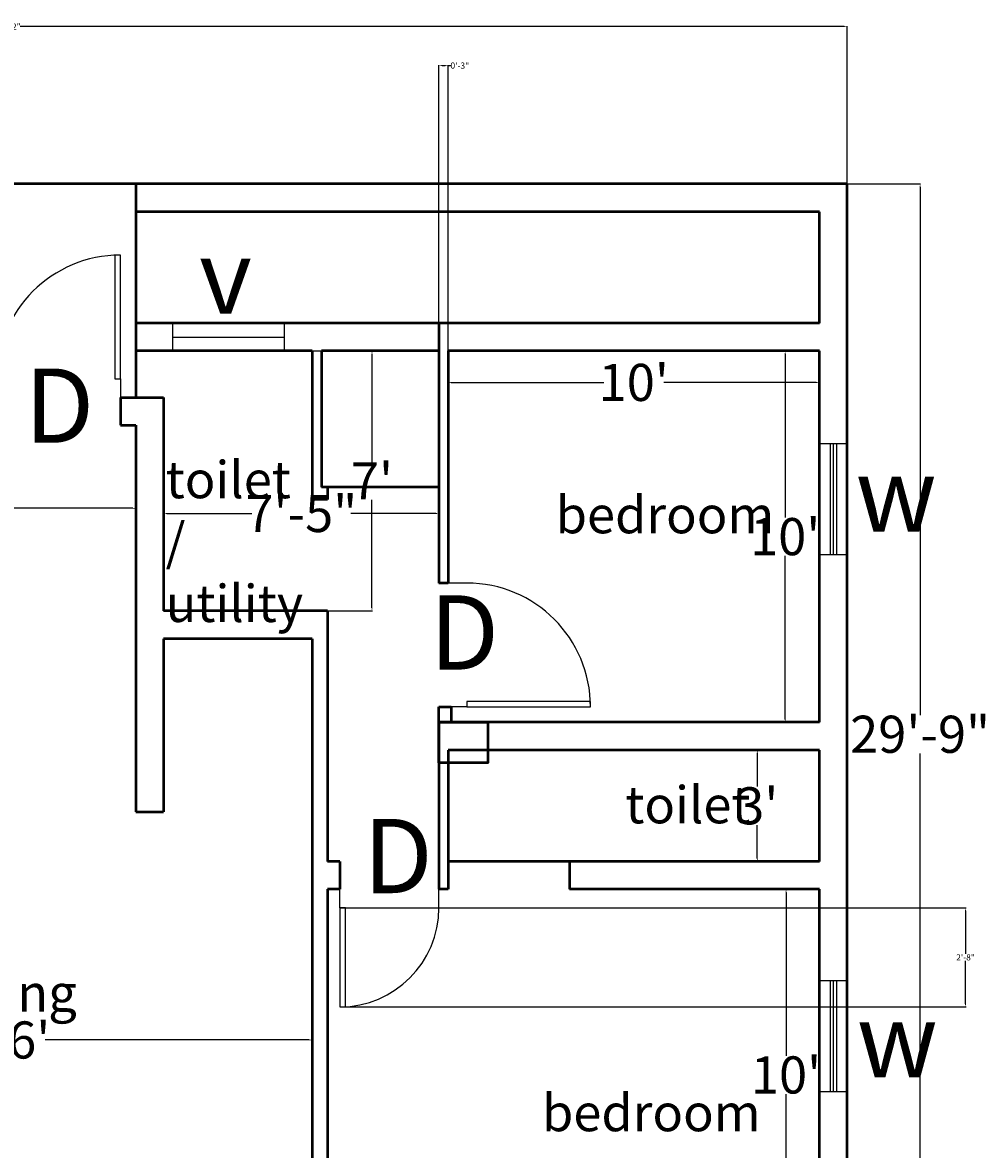
# Model space of a CAD drawing. Units: inches. Extents: x 409 to 7572, y 7 to 725.
# Tile 13 of 38: x 1972 to 2283, y 360 to 725. Entities that reach past the tile are written whole.
import ezdxf

# ---------------------------------------------------------------- set-up
doc = ezdxf.new("R2010")
doc.units = ezdxf.units.IN
doc.header["$MEASUREMENT"] = 0
for name, color, linetype, lineweight in [('A-ANNO-DIMS', 2, 'Continuous', 18), ('A-ANNO-SYMB', 3, 'Continuous', 25), ('A-AREA-IDEN', 7, 'Continuous', 25), ('A-DOOR', 3, 'Continuous', 25), ('A-GLAZ', 4, 'Continuous', 25), ('A-WALL', 7, 'Continuous', 50)]:
    doc.layers.add(name, color=color, linetype=linetype, lineweight=lineweight)
doc.styles.get("Standard").update_dxf_attribs({"font": 'arial.ttf'})
doc.dimstyles.get("Standard").update_dxf_attribs({"dimtxt": 2, "dimasz": 1, "dimexe": 0.18, "dimexo": 0.0625, "dimgap": 0.09, "dimtad": 0, "dimtih": 1, "dimtoh": 1, "dimdec": 0, "dimzin": 0, "dimdsep": 46, "dimlunit": 3, "dimtxsty": 'Standard', "dimcen": 0.09, "dimadec": 0, "dimazin": 0, "dimtfac": 1, "dimtdec": 0, "dimtofl": 0, "dimtmove": 0, "dimatfit": 3, "dimfxl": 1, "dimtolj": 1, "dimtzin": 0, "dimarcsym": 0})

# ---------------------------------------------------------------- blocks, each defined once
blk = doc.blocks.new('*U2')
for p, q in [((0, 0), (0, -6)), ((-40, 0), (-40, -6))]:
    blk.add_line(p, q)
blk.add_lwpolyline([(0, 0), (0, 40), (-1.75, 40), (-1.75, 0)], close=True)
blk.add_arc((0, 0), 40, 90, 180)
blk = doc.blocks.new('*U6')
for p, q in [((0, 0), (0, -6)), ((-40, 0), (-40, -6))]:
    blk.add_line(p, q)
blk.add_lwpolyline([(0, 0), (0, 40), (-1.75, 40), (-1.75, 0)], close=True)
blk.add_arc((0, 0), 40, 90, 180)
blk = doc.blocks.new('*U7')
for p, q in [((0, 0), (0, 6)), ((32, 0), (32, 6))]:
    blk.add_line(p, q)
blk.add_lwpolyline([(0, 0), (0, -32), (1.75, -32), (1.75, 0)], close=True)
blk.add_arc((0, 0), 32, 270, 0)
blk = doc.blocks.new('*D45')
at = {"layer": 'A-ANNO-DIMS', "color": 0, "lineweight": -2, "transparency": 16777216}
for p, q in [((2109.32, 618.47), (2109.32, 608.19)), ((2229.32, 618.47), (2229.32, 608.19)), ((2110.32, 608.37), (2159.61, 608.37)), ((2228.32, 608.37), (2179.03, 608.37))]:
    blk.add_line(p, q, dxfattribs=at)
at = {"layer": 'A-ANNO-DIMS', "color": 0, "transparency": 16777216}
for points in [[(2110.32, 608.54), (2110.32, 608.2), (2109.32, 608.37)], [(2228.32, 608.54), (2228.32, 608.2), (2229.32, 608.37)]]:
    blk.add_solid(points, dxfattribs=at)
at = {"layer": 'DEFPOINTS', "color": 0, "transparency": 16777216}
for p in [(2109.32, 618.53), (2229.32, 618.53), (2109.32, 608.37)]:
    blk.add_point(p, dxfattribs=at)
at = {"layer": 'A-ANNO-DIMS', "color": 0, "transparency": 16777216, "insert": (2169.32, 608.37), "char_height": 2, "attachment_point": 5}
blk.add_mtext("\\A1;{\\H6x;10'}", dxfattribs=at)
blk = doc.blocks.new('*D46')
at = {"layer": 'A-ANNO-DIMS', "color": 0, "lineweight": -2, "transparency": 16777216}
for p, q in [((2229.26, 618.53), (2218.09, 618.53)), ((2218.27, 617.53), (2218.27, 564.75)), ((2218.27, 499.53), (2218.27, 552.31)), ((2229.26, 498.53), (2218.09, 498.53))]:
    blk.add_line(p, q, dxfattribs=at)
at = {"layer": 'A-ANNO-DIMS', "color": 0, "transparency": 16777216}
for points in [[(2218.1, 617.53), (2218.43, 617.53), (2218.27, 618.53)], [(2218.1, 499.53), (2218.43, 499.53), (2218.27, 498.53)]]:
    blk.add_solid(points, dxfattribs=at)
at = {"layer": 'DEFPOINTS', "color": 0, "transparency": 16777216}
for p in [(2218.27, 618.53), (2229.32, 618.53), (2229.32, 498.53)]:
    blk.add_point(p, dxfattribs=at)
at = {"layer": 'A-ANNO-DIMS', "color": 0, "transparency": 16777216, "insert": (2218.27, 558.53), "char_height": 2, "attachment_point": 5}
blk.add_mtext("\\A1;{\\H6x;10'}", dxfattribs=at)
blk = doc.blocks.new('*D47')
at = {"layer": 'A-ANNO-DIMS', "color": 0, "lineweight": -2, "transparency": 16777216}
for p, q in [((2229.26, 444.53), (2218.37, 444.53)), ((2218.55, 443.53), (2218.55, 390.75)), ((2218.55, 325.53), (2218.55, 378.31)), ((2229.26, 324.53), (2218.37, 324.53))]:
    blk.add_line(p, q, dxfattribs=at)
at = {"layer": 'A-ANNO-DIMS', "color": 0, "transparency": 16777216}
for points in [[(2218.39, 443.53), (2218.72, 443.53), (2218.55, 444.53)], [(2218.39, 325.53), (2218.72, 325.53), (2218.55, 324.53)]]:
    blk.add_solid(points, dxfattribs=at)
at = {"layer": 'DEFPOINTS', "color": 0, "transparency": 16777216}
for p in [(2218.55, 444.53), (2229.32, 444.53), (2229.32, 324.53)]:
    blk.add_point(p, dxfattribs=at)
at = {"layer": 'A-ANNO-DIMS', "color": 0, "transparency": 16777216, "insert": (2218.55, 384.53), "char_height": 2, "attachment_point": 5}
blk.add_mtext("\\A1;{\\H6x;10'}", dxfattribs=at)
blk = doc.blocks.new('*D51')
at = {"layer": 'A-ANNO-DIMS', "color": 0, "lineweight": -2, "transparency": 16777216}
for p, q in [((1873.32, 563.4), (1873.32, 567.87)), ((1874.32, 567.69), (1920.68, 567.69)), ((2007.32, 567.69), (1960.96, 567.69)), ((2008.32, 563.4), (2008.32, 567.87))]:
    blk.add_line(p, q, dxfattribs=at)
at = {"layer": 'A-ANNO-DIMS', "color": 0, "transparency": 16777216}
for points in [[(1874.32, 567.86), (1874.32, 567.52), (1873.32, 567.69)], [(2007.32, 567.86), (2007.32, 567.52), (2008.32, 567.69)]]:
    blk.add_solid(points, dxfattribs=at)
at = {"layer": 'DEFPOINTS', "color": 0, "transparency": 16777216}
for p in [(2008.32, 567.69), (1873.32, 563.33), (2008.32, 563.33)]:
    blk.add_point(p, dxfattribs=at)
at = {"layer": 'A-ANNO-DIMS', "color": 0, "transparency": 16777216, "insert": (1940.82, 567.69), "char_height": 2, "attachment_point": 5}
blk.add_mtext('\\A1;{\\H6x;11\'-3"}', dxfattribs=at)
blk = doc.blocks.new('*D52')
at = {"layer": 'A-ANNO-DIMS', "color": 0, "lineweight": -2, "transparency": 16777216}
for p, q in [((1873.32, 403.47), (1873.32, 395.65)), ((2065.32, 403.47), (2065.32, 395.65)), ((1874.32, 395.83), (1959.61, 395.83)), ((2064.32, 395.83), (1979.03, 395.83))]:
    blk.add_line(p, q, dxfattribs=at)
at = {"layer": 'A-ANNO-DIMS', "color": 0, "transparency": 16777216}
for points in [[(1874.32, 396), (1874.32, 395.66), (1873.32, 395.83)], [(2064.32, 396), (2064.32, 395.66), (2065.32, 395.83)]]:
    blk.add_solid(points, dxfattribs=at)
at = {"layer": 'DEFPOINTS', "color": 0, "transparency": 16777216}
for p in [(1873.32, 403.53), (2065.32, 403.53), (2065.32, 395.83)]:
    blk.add_point(p, dxfattribs=at)
at = {"layer": 'A-ANNO-DIMS', "color": 0, "transparency": 16777216, "insert": (1969.32, 395.83), "char_height": 2, "attachment_point": 5}
blk.add_mtext("\\A1;{\\H6x;16'}", dxfattribs=at)
blk = doc.blocks.new('*D57')
at = {"layer": 'A-ANNO-DIMS', "color": 0, "lineweight": -2, "transparency": 16777216}
for p, q in [((2017.32, 568.97), (2017.32, 565.83)), ((2106.32, 568.97), (2106.32, 565.83)), ((2018.32, 566.01), (2045.83, 566.01)), ((2105.32, 566.01), (2077.81, 566.01))]:
    blk.add_line(p, q, dxfattribs=at)
at = {"layer": 'A-ANNO-DIMS', "color": 0, "transparency": 16777216}
for points in [[(2018.32, 566.17), (2018.32, 565.84), (2017.32, 566.01)], [(2105.32, 566.17), (2105.32, 565.84), (2106.32, 566.01)]]:
    blk.add_solid(points, dxfattribs=at)
at = {"layer": 'DEFPOINTS', "color": 0, "transparency": 16777216}
for p in [(2017.32, 569.03), (2106.32, 569.03), (2106.32, 566.01)]:
    blk.add_point(p, dxfattribs=at)
at = {"layer": 'A-ANNO-DIMS', "color": 0, "transparency": 16777216, "insert": (2061.82, 566.01), "char_height": 2, "attachment_point": 5}
blk.add_mtext('\\A1;{\\H6x;7\'-5"}', dxfattribs=at)
blk = doc.blocks.new('*D58')
at = {"layer": 'A-ANNO-DIMS', "color": 0, "lineweight": -2, "transparency": 16777216}
for p, q in [((2036.88, 618.53), (2084.86, 618.53)), ((2084.68, 617.53), (2084.68, 582.62)), ((2084.68, 535.53), (2084.68, 570.44)), ((2036.88, 534.53), (2084.86, 534.53))]:
    blk.add_line(p, q, dxfattribs=at)
at = {"layer": 'A-ANNO-DIMS', "color": 0, "transparency": 16777216}
for points in [[(2084.51, 617.53), (2084.84, 617.53), (2084.68, 618.53)], [(2084.51, 535.53), (2084.84, 535.53), (2084.68, 534.53)]]:
    blk.add_solid(points, dxfattribs=at)
at = {"layer": 'DEFPOINTS', "color": 0, "transparency": 16777216}
for p in [(2036.82, 618.53), (2036.82, 534.53), (2084.68, 534.53)]:
    blk.add_point(p, dxfattribs=at)
at = {"layer": 'A-ANNO-DIMS', "color": 0, "transparency": 16777216, "insert": (2084.68, 576.53), "char_height": 2, "attachment_point": 5}
blk.add_mtext("\\A1;{\\H6x;7'}", dxfattribs=at)
blk = doc.blocks.new('*D60')
at = {"layer": 'A-ANNO-DIMS', "color": 0, "lineweight": -2, "transparency": 16777216}
for p, q in [((2229.26, 489.53), (2209.07, 489.53)), ((2209.25, 488.53), (2209.25, 477.75)), ((2209.25, 454.53), (2209.25, 465.31)), ((2229.26, 453.53), (2209.07, 453.53))]:
    blk.add_line(p, q, dxfattribs=at)
at = {"layer": 'A-ANNO-DIMS', "color": 0, "transparency": 16777216}
for points in [[(2209.08, 488.53), (2209.41, 488.53), (2209.25, 489.53)], [(2209.08, 454.53), (2209.41, 454.53), (2209.25, 453.53)]]:
    blk.add_solid(points, dxfattribs=at)
at = {"layer": 'DEFPOINTS', "color": 0, "transparency": 16777216}
for p in [(2229.32, 489.53), (2209.25, 453.53), (2229.32, 453.53)]:
    blk.add_point(p, dxfattribs=at)
at = {"layer": 'A-ANNO-DIMS', "color": 0, "transparency": 16777216, "insert": (2209.25, 471.53), "char_height": 2, "attachment_point": 5}
blk.add_mtext("\\A1;{\\H6x;3'}", dxfattribs=at)
blk = doc.blocks.new('*D62')
at = {"layer": 'A-ANNO-DIMS', "color": 0, "lineweight": -2, "transparency": 16777216}
for p, q in [((1696.32, 672.59), (1696.32, 723.56)), ((1697.32, 723.38), (1963.75, 723.38)), ((2237.32, 723.38), (1970.88, 723.38)), ((2238.32, 672.59), (2238.32, 723.56))]:
    blk.add_line(p, q, dxfattribs=at)
at = {"layer": 'A-ANNO-DIMS', "color": 0, "transparency": 16777216}
for points in [[(1697.32, 723.55), (1697.32, 723.22), (1696.32, 723.38)], [(2237.32, 723.55), (2237.32, 723.22), (2238.32, 723.38)]]:
    blk.add_solid(points, dxfattribs=at)
at = {"layer": 'DEFPOINTS', "color": 0, "transparency": 16777216}
for p in [(1696.32, 723.38), (1696.32, 672.53), (2238.32, 672.53)]:
    blk.add_point(p, dxfattribs=at)
at = {"layer": 'A-ANNO-DIMS', "color": 0, "transparency": 16777216, "insert": (1967.32, 723.38), "char_height": 2, "attachment_point": 5}
blk.add_mtext('\\A1;45\'-2"', dxfattribs=at)
blk = doc.blocks.new('*D64')
at = {"layer": 'A-ANNO-DIMS', "color": 0, "lineweight": -2, "transparency": 16777216}
for p, q in [((2238.38, 672.53), (2262.07, 672.53)), ((2261.89, 671.53), (2261.89, 500.86)), ((2261.89, 316.53), (2261.89, 488.43)), ((2238.38, 315.53), (2262.07, 315.53))]:
    blk.add_line(p, q, dxfattribs=at)
at = {"layer": 'A-ANNO-DIMS', "color": 0, "transparency": 16777216}
for points in [[(2261.72, 671.53), (2262.05, 671.53), (2261.89, 672.53)], [(2261.72, 316.53), (2262.05, 316.53), (2261.89, 315.53)]]:
    blk.add_solid(points, dxfattribs=at)
at = {"layer": 'DEFPOINTS', "color": 0, "transparency": 16777216}
for p in [(2238.32, 672.53), (2261.89, 672.53), (2238.32, 315.53)]:
    blk.add_point(p, dxfattribs=at)
at = {"layer": 'A-ANNO-DIMS', "color": 0, "transparency": 16777216, "insert": (2261.89, 494.65), "char_height": 2, "attachment_point": 5}
blk.add_mtext('\\A1;{\\H6x;29\'-9"}', dxfattribs=at)
blk = doc.blocks.new('WIN-36')
for p, q in [((1699.82, 514.65), (1699.82, 478.65)), ((1700.82, 514.65), (1700.82, 478.65)), ((1701.82, 514.65), (1701.82, 478.65))]:
    blk.add_line(p, q)
blk.add_lwpolyline([(1705.32, 514.65), (1705.32, 478.65), (1696.32, 478.65), (1696.32, 514.65)], close=True)
blk = doc.blocks.new('VENT-36')
blk.add_line((5633.28, 355.73), (5633.28, 391.73))
blk.add_lwpolyline([(5628.78, 355.73), (5628.78, 391.73), (5637.78, 391.73), (5637.78, 355.73)], close=True)
blk = doc.blocks.new('*D180')
at = {"layer": 'A-ANNO-DIMS', "color": 0, "lineweight": -2, "transparency": 16777216}
for p, q in [((2106.32, 627.59), (2106.32, 710.96)), ((2107.32, 710.78), (2108.32, 710.78)), ((2109.32, 618.59), (2109.32, 710.96)), ((2109.32, 710.78), (2110.32, 710.78))]:
    blk.add_line(p, q, dxfattribs=at)
at = {"layer": 'A-ANNO-DIMS', "color": 0, "transparency": 16777216}
for points in [[(2107.32, 710.95), (2107.32, 710.61), (2106.32, 710.78)], [(2108.32, 710.95), (2108.32, 710.61), (2109.32, 710.78)]]:
    blk.add_solid(points, dxfattribs=at)
at = {"layer": 'DEFPOINTS', "color": 0, "transparency": 16777216}
for p in [(2109.32, 710.78), (2106.32, 627.53), (2109.32, 618.53)]:
    blk.add_point(p, dxfattribs=at)
at = {"layer": 'A-ANNO-DIMS', "color": 0, "transparency": 16777216, "insert": (2113.07, 710.78), "char_height": 2, "attachment_point": 5}
blk.add_mtext('\\A1;0\'-3"', dxfattribs=at)
blk = doc.blocks.new('*D181')
at = {"layer": 'A-ANNO-DIMS', "color": 0, "lineweight": -2, "transparency": 16777216}
for p, q in [((2074.38, 438.53), (2276.75, 438.53)), ((2276.57, 437.53), (2276.57, 423.64)), ((2276.57, 407.53), (2276.57, 421.42)), ((2074.38, 406.53), (2276.75, 406.53))]:
    blk.add_line(p, q, dxfattribs=at)
at = {"layer": 'A-ANNO-DIMS', "color": 0, "transparency": 16777216}
for points in [[(2276.4, 437.53), (2276.74, 437.53), (2276.57, 438.53)], [(2276.4, 407.53), (2276.74, 407.53), (2276.57, 406.53)]]:
    blk.add_solid(points, dxfattribs=at)
at = {"layer": 'DEFPOINTS', "color": 0, "transparency": 16777216}
for p in [(2074.32, 438.53), (2074.32, 406.53), (2276.57, 406.53)]:
    blk.add_point(p, dxfattribs=at)
at = {"layer": 'A-ANNO-DIMS', "color": 0, "transparency": 16777216, "insert": (2276.57, 422.53), "char_height": 2, "attachment_point": 5}
blk.add_mtext('\\A1;2\'-8"', dxfattribs=at)

msp = doc.modelspace()

# ---------------------------------------------------------------- linework, layer by layer
at = {"layer": 'A-WALL'}
for p, q in [((2238.32, 672.53), (1696.32, 672.53)), ((2008.32, 672.53), (2008.32, 603.53)), ((2238.32, 315.53), (2238.32, 672.53)), ((2229.32, 663.53), (2008.32, 663.53)), ((2229.32, 627.53), (2229.32, 663.53)), ((2229.32, 627.53), (2008.32, 627.53)), ((2106.32, 627.53), (2106.32, 543.53)), ((2065.32, 618.53), (2008.32, 618.53)), ((2065.32, 618.53), (2065.32, 570.53)), ((2106.32, 618.53), (2068.32, 618.53)), ((2068.32, 618.53), (2068.32, 574.53)), ((2229.32, 618.53), (2109.32, 618.53)), ((2109.32, 618.53), (2109.32, 543.53)), ((2229.32, 498.53), (2229.32, 618.53)), ((2003.32, 603.53), (2017.32, 603.53)), ((2003.32, 603.53), (2003.32, 594.53)), ((2017.32, 603.53), (2017.32, 534.53)), ((2003.32, 594.53), (2008.32, 594.53)), ((2106.32, 574.53), (2068.32, 574.53)), ((2070.32, 574.53), (2070.32, 570.53)), ((2070.32, 570.53), (2065.32, 570.53)), ((2109.32, 543.53), (2106.32, 543.53)), ((2070.32, 534.53), (2017.32, 534.53)), ((2070.32, 534.53), (2070.32, 453.53)), ((2065.32, 525.53), (2017.32, 525.53)), ((2017.32, 525.53), (2017.32, 469.53)), ((2065.32, 525.53), (2065.32, 337.53)), ((2106.32, 498.53), (2106.32, 503.53)), ((2106.32, 503.53), (2110.32, 503.53)), ((2110.32, 503.53), (2110.32, 498.53)), ((2229.32, 498.53), (2106.32, 498.53)), ((2106.32, 498.53), (2106.32, 444.53)), ((2065.32, 489.53), (2065.32, 337.53)), ((2229.32, 489.53), (2109.32, 489.53)), ((2109.32, 489.53), (2109.32, 444.53)), ((2229.32, 453.53), (2229.32, 489.53)), ((2008.32, 469.53), (2017.32, 469.53)), ((2074.32, 453.53), (2070.32, 453.53)), ((2074.32, 453.53), (2074.32, 444.53)), ((2229.32, 453.53), (2109.32, 453.53)), ((2148.51, 453.53), (2148.51, 444.53)), ((2074.32, 444.53), (2070.32, 444.53)), ((2070.32, 444.53), (2070.32, 324.53)), ((2109.32, 444.53), (2106.32, 444.53)), ((2109.32, 444.53), (2106.32, 444.53)), ((2229.32, 444.53), (2148.51, 444.53)), ((2229.32, 324.53), (2229.32, 444.53))]:
    msp.add_line(p, q, dxfattribs=at)
msp.add_lwpolyline([(2008.32, 594.53), (2008.32, 525.53), (2008.32, 469.53)], dxfattribs=at)
msp.add_lwpolyline([(2106.32, 498.53), (2122.18, 498.53), (2122.18, 485.36), (2106.32, 485.36)], close=True, dxfattribs=at)

# ---------------------------------------------------------------- block references
at = {"layer": 'A-DOOR'}
for name, p in [('*U2', (2003.32, 609.53)), ('*U7', (2074.32, 438.53))]:
    msp.add_blockref(name, p, dxfattribs=at)
at = {"layer": 'A-DOOR', "rotation": 270}
msp.add_blockref('*U6', (2115.32, 503.53), dxfattribs=at)
at = {"layer": 'A-GLAZ', "rotation": 269.9999999999996}
msp.add_blockref('VENT-36', (1664.51, 6256.31), dxfattribs=at)
at = {"layer": 'A-GLAZ'}
for p in [(533, 73.99), (533, -99.57)]:
    msp.add_blockref('WIN-36', p, dxfattribs=at)

# ---------------------------------------------------------------- texts
at = {"layer": 'A-ANNO-SYMB', "char_height": 24, "attachment_point": 1}
for s, width, insert in [('v', 18.2582, (2028.79, 654.55)), ('D', 19.1972, (1972.35, 612.87)), ('w', 18.2582, (2241, 584.1)), ('D', 19.1972, (2103.25, 539.54)), ('D', 19.1972, (2081.82, 467.28)), ('w', 18.2582, (2241.38, 407.81))]:
    msp.add_mtext_dynamic_manual_height_columns(s, width=width, gutter_width=1, heights=[0], dxfattribs=dict(at, insert=insert))
at = {"layer": 'A-AREA-IDEN', "char_height": 12, "attachment_point": 1}
for s, width, insert in [('toilet / utility', 49.2946, (2017.97, 582.94)), ('bedroom', 40.9017, (2144.07, 571.6)), ('toilet', 49.2946, (2166.57, 477.86)), ('Dining ', 67.5069, (1939.75, 417.03)), ('bedroom', 40.9017, (2139.65, 378.34))]:
    msp.add_mtext_dynamic_manual_height_columns(s, width=width, gutter_width=1, heights=[0], dxfattribs=dict(at, insert=insert))

# ---------------------------------------------------------------- dimensions: what is measured, and where the dimension line sits
at = {"layer": 'A-ANNO-DIMS'}
for base, p1, p2, override, picture, middle in [((1696.32, 723.38), (2238.32, 672.53), (1696.32, 672.53), {"dimclrd": 0, "dimclre": 0, "dimclrt": 0}, '*D62', (1967.32, 723.38)), ((2109.32, 710.78), (2106.32, 627.53), (2109.32, 618.53), {"dimdec": 1, "dimlfac": 1, "dimrnd": 0, "dimzin": 1, "dimdsep": 46, "dimlunit": 4, "dimfrac": 2}, '*D180', (2113.07, 710.78))]:
    dim = msp.add_linear_dim(base=base, p1=p1, p2=p2, dimstyle='Standard', override=override, dxfattribs=at)
    dim.commit()
    dim.dimension.update_dxf_attribs({"geometry": picture, "text_midpoint": middle})
dim = msp.add_linear_dim(base=(2261.89, 672.53), p1=(2238.32, 315.53), p2=(2238.32, 672.53), angle=90, text='{\\H6x;<>}', dimstyle='Standard', override={"dimclrd": 0, "dimclre": 0, "dimclrt": 0}, dxfattribs=at)
dim.commit()
dim.dimension.update_dxf_attribs({"geometry": '*D64', "text_midpoint": (2261.89, 494.65), "dimtype": 160})
for base, p1, p2, picture, middle in [((2084.68, 534.53), (2036.82, 618.53), (2036.82, 534.53), '*D58', (2084.68, 576.53)), ((2218.27, 618.53), (2229.32, 498.53), (2229.32, 618.53), '*D46', (2218.27, 558.53)), ((2209.25, 453.53), (2229.32, 489.53), (2229.32, 453.53), '*D60', (2209.25, 471.53)), ((2218.55, 444.53), (2229.32, 324.53), (2229.32, 444.53), '*D47', (2218.55, 384.53))]:
    dim = msp.add_linear_dim(base=base, p1=p1, p2=p2, angle=90, text='{\\H6x;<>}', dimstyle='Standard', override={"dimclrd": 0, "dimclre": 0, "dimclrt": 0}, dxfattribs=at)
    dim.commit()
    dim.dimension.update_dxf_attribs({"geometry": picture, "text_midpoint": middle})
for base, p1, p2, picture, middle in [((2109.32, 608.37), (2229.32, 618.53), (2109.32, 618.53), '*D45', (2169.32, 608.37)), ((2008.32, 567.69), (1873.32, 563.33), (2008.32, 563.33), '*D51', (1940.82, 567.69)), ((2106.32, 566.01), (2017.32, 569.03), (2106.32, 569.03), '*D57', (2061.82, 566.01))]:
    dim = msp.add_linear_dim(base=base, p1=p1, p2=p2, text='{\\H6x;<>}', dimstyle='Standard', override={"dimclrd": 0, "dimclre": 0, "dimclrt": 0}, dxfattribs=at)
    dim.commit()
    dim.dimension.update_dxf_attribs({"geometry": picture, "text_midpoint": middle})
dim = msp.add_linear_dim(base=(2276.57, 406.53), p1=(2074.32, 438.53), p2=(2074.32, 406.53), angle=90, dimstyle='Standard', override={"dimdec": 1, "dimlfac": 1, "dimrnd": 0, "dimzin": 1, "dimdsep": 46, "dimlunit": 4, "dimfrac": 2}, dxfattribs=at)
dim.commit()
dim.dimension.update_dxf_attribs({"geometry": '*D181', "text_midpoint": (2276.57, 422.53)})
dim = msp.add_linear_dim(base=(2065.32, 395.83), p1=(1873.32, 403.53), p2=(2065.32, 403.53), text='{\\H6x;<>}', dimstyle='Standard', override={"dimclrd": 0, "dimclre": 0, "dimclrt": 0}, dxfattribs=at)
dim.commit()
dim.dimension.update_dxf_attribs({"geometry": '*D52', "text_midpoint": (1969.32, 395.83), "dimtype": 160})

doc.saveas('drawing.dxf')
